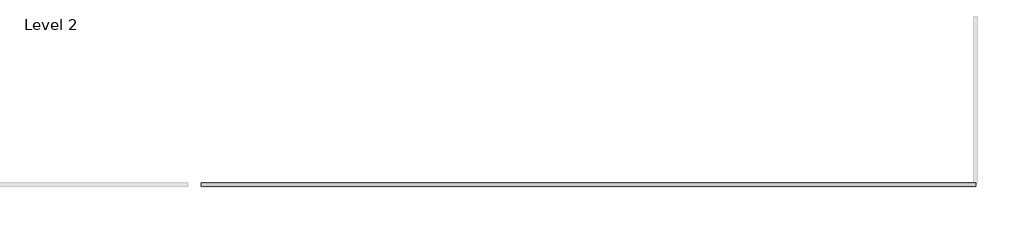
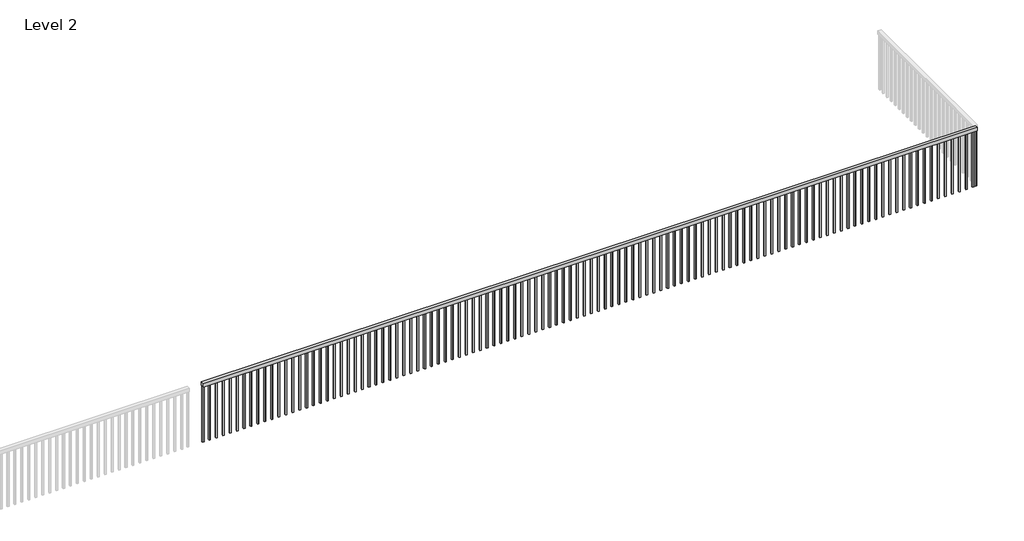
# One storey, part 2 of 5: 1 railing.
"""IFC4 building model written with IfcOpenShell, lengths in millimetres."""

from ifc_helpers import new_model, si_unit, frame, origin, place, context, project, spatial, polyline, outline, extrude, element, save

model = new_model("IFC4")

# Units and contexts
model_context = context("Model", 3, world=origin())
ifc_project = project(units=[si_unit("LENGTHUNIT", "METRE", prefix="MILLI")], contexts=[model_context])

# Site, building, storey
site = spatial("IfcSite", under=ifc_project)
building = spatial("IfcBuilding", under=site)
storey = spatial("IfcBuildingStorey", under=building, Name="Level 2", Elevation=3048.0)

# Railing
placement = place(None, origin())
element("IfcRailing", 1, ObjectType="Handrail - Rectangular", at=placement, inside=storey, context=model_context, shape_type="SweptSolid", body=[
    extrude(outline(polyline([(2981.3361222, -12911.7749501), (2981.3361222, -12860.9749501), (14309.7361222, -12860.9749501), (14309.7361222, -12911.7749501), (2981.3361222, -12911.7749501)])), frame((0.0, 0.0, 3911.6), z_axis=(0.0, 0.0, 1.0), x_axis=(1.0, 0.0, 0.0)), (0.0, 0.0, 1.0), 50.8),
    extrude(outline(polyline([(14249.4111222, -12895.8999501), (14249.4111222, -12876.8499501), (14268.4611222, -12876.8499501), (14268.4611222, -12895.8999501), (14249.4111222, -12895.8999501)])), frame((0.0, 0.0, 3048.0), z_axis=(0.0, 0.0, 1.0), x_axis=(1.0, 0.0, 0.0)), (0.0, 0.0, 1.0), 863.6),
    extrude(outline(polyline([(14147.8111222, -12895.8999501), (14147.8111222, -12876.8499501), (14166.8611222, -12876.8499501), (14166.8611222, -12895.8999501), (14147.8111222, -12895.8999501)])), frame((0.0, 0.0, 3048.0), z_axis=(0.0, 0.0, 1.0), x_axis=(1.0, 0.0, 0.0)), (0.0, 0.0, 1.0), 863.6),
    extrude(outline(polyline([(14046.2111222, -12895.8999501), (14046.2111222, -12876.8499501), (14065.2611222, -12876.8499501), (14065.2611222, -12895.8999501), (14046.2111222, -12895.8999501)])), frame((0.0, 0.0, 3048.0), z_axis=(0.0, 0.0, 1.0), x_axis=(1.0, 0.0, 0.0)), (0.0, 0.0, 1.0), 863.6),
    extrude(outline(polyline([(13944.6111222, -12895.8999501), (13944.6111222, -12876.8499501), (13963.6611222, -12876.8499501), (13963.6611222, -12895.8999501), (13944.6111222, -12895.8999501)])), frame((0.0, 0.0, 3048.0), z_axis=(0.0, 0.0, 1.0), x_axis=(1.0, 0.0, 0.0)), (0.0, 0.0, 1.0), 863.6),
    extrude(outline(polyline([(13843.0111222, -12895.8999501), (13843.0111222, -12876.8499501), (13862.0611222, -12876.8499501), (13862.0611222, -12895.8999501), (13843.0111222, -12895.8999501)])), frame((0.0, 0.0, 3048.0), z_axis=(0.0, 0.0, 1.0), x_axis=(1.0, 0.0, 0.0)), (0.0, 0.0, 1.0), 863.6),
    extrude(outline(polyline([(13741.4111222, -12895.8999501), (13741.4111222, -12876.8499501), (13760.4611222, -12876.8499501), (13760.4611222, -12895.8999501), (13741.4111222, -12895.8999501)])), frame((0.0, 0.0, 3048.0), z_axis=(0.0, 0.0, 1.0), x_axis=(1.0, 0.0, 0.0)), (0.0, 0.0, 1.0), 863.6),
    extrude(outline(polyline([(13639.8111222, -12895.8999501), (13639.8111222, -12876.8499501), (13658.8611222, -12876.8499501), (13658.8611222, -12895.8999501), (13639.8111222, -12895.8999501)])), frame((0.0, 0.0, 3048.0), z_axis=(0.0, 0.0, 1.0), x_axis=(1.0, 0.0, 0.0)), (0.0, 0.0, 1.0), 863.6),
    extrude(outline(polyline([(13538.2111222, -12895.8999501), (13538.2111222, -12876.8499501), (13557.2611222, -12876.8499501), (13557.2611222, -12895.8999501), (13538.2111222, -12895.8999501)])), frame((0.0, 0.0, 3048.0), z_axis=(0.0, 0.0, 1.0), x_axis=(1.0, 0.0, 0.0)), (0.0, 0.0, 1.0), 863.6),
    extrude(outline(polyline([(13436.6111222, -12895.8999501), (13436.6111222, -12876.8499501), (13455.6611222, -12876.8499501), (13455.6611222, -12895.8999501), (13436.6111222, -12895.8999501)])), frame((0.0, 0.0, 3048.0), z_axis=(0.0, 0.0, 1.0), x_axis=(1.0, 0.0, 0.0)), (0.0, 0.0, 1.0), 863.6),
    extrude(outline(polyline([(13335.0111222, -12895.8999501), (13335.0111222, -12876.8499501), (13354.0611222, -12876.8499501), (13354.0611222, -12895.8999501), (13335.0111222, -12895.8999501)])), frame((0.0, 0.0, 3048.0), z_axis=(0.0, 0.0, 1.0), x_axis=(1.0, 0.0, 0.0)), (0.0, 0.0, 1.0), 863.6),
    extrude(outline(polyline([(13233.4111222, -12895.8999501), (13233.4111222, -12876.8499501), (13252.4611222, -12876.8499501), (13252.4611222, -12895.8999501), (13233.4111222, -12895.8999501)])), frame((0.0, 0.0, 3048.0), z_axis=(0.0, 0.0, 1.0), x_axis=(1.0, 0.0, 0.0)), (0.0, 0.0, 1.0), 863.6),
    extrude(outline(polyline([(13131.8111222, -12895.8999501), (13131.8111222, -12876.8499501), (13150.8611222, -12876.8499501), (13150.8611222, -12895.8999501), (13131.8111222, -12895.8999501)])), frame((0.0, 0.0, 3048.0), z_axis=(0.0, 0.0, 1.0), x_axis=(1.0, 0.0, 0.0)), (0.0, 0.0, 1.0), 863.6),
    extrude(outline(polyline([(13030.2111222, -12895.8999501), (13030.2111222, -12876.8499501), (13049.2611222, -12876.8499501), (13049.2611222, -12895.8999501), (13030.2111222, -12895.8999501)])), frame((0.0, 0.0, 3048.0), z_axis=(0.0, 0.0, 1.0), x_axis=(1.0, 0.0, 0.0)), (0.0, 0.0, 1.0), 863.6),
    extrude(outline(polyline([(12928.6111222, -12895.8999501), (12928.6111222, -12876.8499501), (12947.6611222, -12876.8499501), (12947.6611222, -12895.8999501), (12928.6111222, -12895.8999501)])), frame((0.0, 0.0, 3048.0), z_axis=(0.0, 0.0, 1.0), x_axis=(1.0, 0.0, 0.0)), (0.0, 0.0, 1.0), 863.6),
    extrude(outline(polyline([(12827.0111222, -12895.8999501), (12827.0111222, -12876.8499501), (12846.0611222, -12876.8499501), (12846.0611222, -12895.8999501), (12827.0111222, -12895.8999501)])), frame((0.0, 0.0, 3048.0), z_axis=(0.0, 0.0, 1.0), x_axis=(1.0, 0.0, 0.0)), (0.0, 0.0, 1.0), 863.6),
    extrude(outline(polyline([(12725.4111222, -12895.8999501), (12725.4111222, -12876.8499501), (12744.4611222, -12876.8499501), (12744.4611222, -12895.8999501), (12725.4111222, -12895.8999501)])), frame((0.0, 0.0, 3048.0), z_axis=(0.0, 0.0, 1.0), x_axis=(1.0, 0.0, 0.0)), (0.0, 0.0, 1.0), 863.6),
    extrude(outline(polyline([(12623.8111222, -12895.8999501), (12623.8111222, -12876.8499501), (12642.8611222, -12876.8499501), (12642.8611222, -12895.8999501), (12623.8111222, -12895.8999501)])), frame((0.0, 0.0, 3048.0), z_axis=(0.0, 0.0, 1.0), x_axis=(1.0, 0.0, 0.0)), (0.0, 0.0, 1.0), 863.6),
    extrude(outline(polyline([(12522.2111222, -12895.8999501), (12522.2111222, -12876.8499501), (12541.2611222, -12876.8499501), (12541.2611222, -12895.8999501), (12522.2111222, -12895.8999501)])), frame((0.0, 0.0, 3048.0), z_axis=(0.0, 0.0, 1.0), x_axis=(1.0, 0.0, 0.0)), (0.0, 0.0, 1.0), 863.6),
    extrude(outline(polyline([(12420.6111222, -12895.8999501), (12420.6111222, -12876.8499501), (12439.6611222, -12876.8499501), (12439.6611222, -12895.8999501), (12420.6111222, -12895.8999501)])), frame((0.0, 0.0, 3048.0), z_axis=(0.0, 0.0, 1.0), x_axis=(1.0, 0.0, 0.0)), (0.0, 0.0, 1.0), 863.6),
    extrude(outline(polyline([(12319.0111222, -12895.8999501), (12319.0111222, -12876.8499501), (12338.0611222, -12876.8499501), (12338.0611222, -12895.8999501), (12319.0111222, -12895.8999501)])), frame((0.0, 0.0, 3048.0), z_axis=(0.0, 0.0, 1.0), x_axis=(1.0, 0.0, 0.0)), (0.0, 0.0, 1.0), 863.6),
    extrude(outline(polyline([(12217.4111222, -12895.8999501), (12217.4111222, -12876.8499501), (12236.4611222, -12876.8499501), (12236.4611222, -12895.8999501), (12217.4111222, -12895.8999501)])), frame((0.0, 0.0, 3048.0), z_axis=(0.0, 0.0, 1.0), x_axis=(1.0, 0.0, 0.0)), (0.0, 0.0, 1.0), 863.6),
    extrude(outline(polyline([(12115.8111222, -12895.8999501), (12115.8111222, -12876.8499501), (12134.8611222, -12876.8499501), (12134.8611222, -12895.8999501), (12115.8111222, -12895.8999501)])), frame((0.0, 0.0, 3048.0), z_axis=(0.0, 0.0, 1.0), x_axis=(1.0, 0.0, 0.0)), (0.0, 0.0, 1.0), 863.6),
    extrude(outline(polyline([(12014.2111222, -12895.8999501), (12014.2111222, -12876.8499501), (12033.2611222, -12876.8499501), (12033.2611222, -12895.8999501), (12014.2111222, -12895.8999501)])), frame((0.0, 0.0, 3048.0), z_axis=(0.0, 0.0, 1.0), x_axis=(1.0, 0.0, 0.0)), (0.0, 0.0, 1.0), 863.6),
    extrude(outline(polyline([(11912.6111222, -12895.8999501), (11912.6111222, -12876.8499501), (11931.6611222, -12876.8499501), (11931.6611222, -12895.8999501), (11912.6111222, -12895.8999501)])), frame((0.0, 0.0, 3048.0), z_axis=(0.0, 0.0, 1.0), x_axis=(1.0, 0.0, 0.0)), (0.0, 0.0, 1.0), 863.6),
    extrude(outline(polyline([(11811.0111222, -12895.8999501), (11811.0111222, -12876.8499501), (11830.0611222, -12876.8499501), (11830.0611222, -12895.8999501), (11811.0111222, -12895.8999501)])), frame((0.0, 0.0, 3048.0), z_axis=(0.0, 0.0, 1.0), x_axis=(1.0, 0.0, 0.0)), (0.0, 0.0, 1.0), 863.6),
    extrude(outline(polyline([(11709.4111222, -12895.8999501), (11709.4111222, -12876.8499501), (11728.4611222, -12876.8499501), (11728.4611222, -12895.8999501), (11709.4111222, -12895.8999501)])), frame((0.0, 0.0, 3048.0), z_axis=(0.0, 0.0, 1.0), x_axis=(1.0, 0.0, 0.0)), (0.0, 0.0, 1.0), 863.6),
    extrude(outline(polyline([(11607.8111222, -12895.8999501), (11607.8111222, -12876.8499501), (11626.8611222, -12876.8499501), (11626.8611222, -12895.8999501), (11607.8111222, -12895.8999501)])), frame((0.0, 0.0, 3048.0), z_axis=(0.0, 0.0, 1.0), x_axis=(1.0, 0.0, 0.0)), (0.0, 0.0, 1.0), 863.6),
    extrude(outline(polyline([(11506.2111222, -12895.8999501), (11506.2111222, -12876.8499501), (11525.2611222, -12876.8499501), (11525.2611222, -12895.8999501), (11506.2111222, -12895.8999501)])), frame((0.0, 0.0, 3048.0), z_axis=(0.0, 0.0, 1.0), x_axis=(1.0, 0.0, 0.0)), (0.0, 0.0, 1.0), 863.6),
    extrude(outline(polyline([(11404.6111222, -12895.8999501), (11404.6111222, -12876.8499501), (11423.6611222, -12876.8499501), (11423.6611222, -12895.8999501), (11404.6111222, -12895.8999501)])), frame((0.0, 0.0, 3048.0), z_axis=(0.0, 0.0, 1.0), x_axis=(1.0, 0.0, 0.0)), (0.0, 0.0, 1.0), 863.6),
    extrude(outline(polyline([(11303.0111222, -12895.8999501), (11303.0111222, -12876.8499501), (11322.0611222, -12876.8499501), (11322.0611222, -12895.8999501), (11303.0111222, -12895.8999501)])), frame((0.0, 0.0, 3048.0), z_axis=(0.0, 0.0, 1.0), x_axis=(1.0, 0.0, 0.0)), (0.0, 0.0, 1.0), 863.6),
    extrude(outline(polyline([(11201.4111222, -12895.8999501), (11201.4111222, -12876.8499501), (11220.4611222, -12876.8499501), (11220.4611222, -12895.8999501), (11201.4111222, -12895.8999501)])), frame((0.0, 0.0, 3048.0), z_axis=(0.0, 0.0, 1.0), x_axis=(1.0, 0.0, 0.0)), (0.0, 0.0, 1.0), 863.6),
    extrude(outline(polyline([(11099.8111222, -12895.8999501), (11099.8111222, -12876.8499501), (11118.8611222, -12876.8499501), (11118.8611222, -12895.8999501), (11099.8111222, -12895.8999501)])), frame((0.0, 0.0, 3048.0), z_axis=(0.0, 0.0, 1.0), x_axis=(1.0, 0.0, 0.0)), (0.0, 0.0, 1.0), 863.6),
    extrude(outline(polyline([(10998.2111222, -12895.8999501), (10998.2111222, -12876.8499501), (11017.2611222, -12876.8499501), (11017.2611222, -12895.8999501), (10998.2111222, -12895.8999501)])), frame((0.0, 0.0, 3048.0), z_axis=(0.0, 0.0, 1.0), x_axis=(1.0, 0.0, 0.0)), (0.0, 0.0, 1.0), 863.6),
    extrude(outline(polyline([(10896.6111222, -12895.8999501), (10896.6111222, -12876.8499501), (10915.6611222, -12876.8499501), (10915.6611222, -12895.8999501), (10896.6111222, -12895.8999501)])), frame((0.0, 0.0, 3048.0), z_axis=(0.0, 0.0, 1.0), x_axis=(1.0, 0.0, 0.0)), (0.0, 0.0, 1.0), 863.6),
    extrude(outline(polyline([(10795.0111222, -12895.8999501), (10795.0111222, -12876.8499501), (10814.0611222, -12876.8499501), (10814.0611222, -12895.8999501), (10795.0111222, -12895.8999501)])), frame((0.0, 0.0, 3048.0), z_axis=(0.0, 0.0, 1.0), x_axis=(1.0, 0.0, 0.0)), (0.0, 0.0, 1.0), 863.6),
    extrude(outline(polyline([(10693.4111222, -12895.8999501), (10693.4111222, -12876.8499501), (10712.4611222, -12876.8499501), (10712.4611222, -12895.8999501), (10693.4111222, -12895.8999501)])), frame((0.0, 0.0, 3048.0), z_axis=(0.0, 0.0, 1.0), x_axis=(1.0, 0.0, 0.0)), (0.0, 0.0, 1.0), 863.6),
    extrude(outline(polyline([(10591.8111222, -12895.8999501), (10591.8111222, -12876.8499501), (10610.8611222, -12876.8499501), (10610.8611222, -12895.8999501), (10591.8111222, -12895.8999501)])), frame((0.0, 0.0, 3048.0), z_axis=(0.0, 0.0, 1.0), x_axis=(1.0, 0.0, 0.0)), (0.0, 0.0, 1.0), 863.6),
    extrude(outline(polyline([(10490.2111222, -12895.8999501), (10490.2111222, -12876.8499501), (10509.2611222, -12876.8499501), (10509.2611222, -12895.8999501), (10490.2111222, -12895.8999501)])), frame((0.0, 0.0, 3048.0), z_axis=(0.0, 0.0, 1.0), x_axis=(1.0, 0.0, 0.0)), (0.0, 0.0, 1.0), 863.6),
    extrude(outline(polyline([(10388.6111222, -12895.8999501), (10388.6111222, -12876.8499501), (10407.6611222, -12876.8499501), (10407.6611222, -12895.8999501), (10388.6111222, -12895.8999501)])), frame((0.0, 0.0, 3048.0), z_axis=(0.0, 0.0, 1.0), x_axis=(1.0, 0.0, 0.0)), (0.0, 0.0, 1.0), 863.6),
    extrude(outline(polyline([(10287.0111222, -12895.8999501), (10287.0111222, -12876.8499501), (10306.0611222, -12876.8499501), (10306.0611222, -12895.8999501), (10287.0111222, -12895.8999501)])), frame((0.0, 0.0, 3048.0), z_axis=(0.0, 0.0, 1.0), x_axis=(1.0, 0.0, 0.0)), (0.0, 0.0, 1.0), 863.6),
    extrude(outline(polyline([(10185.4111222, -12895.8999501), (10185.4111222, -12876.8499501), (10204.4611222, -12876.8499501), (10204.4611222, -12895.8999501), (10185.4111222, -12895.8999501)])), frame((0.0, 0.0, 3048.0), z_axis=(0.0, 0.0, 1.0), x_axis=(1.0, 0.0, 0.0)), (0.0, 0.0, 1.0), 863.6),
    extrude(outline(polyline([(10083.8111222, -12895.8999501), (10083.8111222, -12876.8499501), (10102.8611222, -12876.8499501), (10102.8611222, -12895.8999501), (10083.8111222, -12895.8999501)])), frame((0.0, 0.0, 3048.0), z_axis=(0.0, 0.0, 1.0), x_axis=(1.0, 0.0, 0.0)), (0.0, 0.0, 1.0), 863.6),
    extrude(outline(polyline([(9982.2111222, -12895.8999501), (9982.2111222, -12876.8499501), (10001.2611222, -12876.8499501), (10001.2611222, -12895.8999501), (9982.2111222, -12895.8999501)])), frame((0.0, 0.0, 3048.0), z_axis=(0.0, 0.0, 1.0), x_axis=(1.0, 0.0, 0.0)), (0.0, 0.0, 1.0), 863.6),
    extrude(outline(polyline([(9880.6111222, -12895.8999501), (9880.6111222, -12876.8499501), (9899.6611222, -12876.8499501), (9899.6611222, -12895.8999501), (9880.6111222, -12895.8999501)])), frame((0.0, 0.0, 3048.0), z_axis=(0.0, 0.0, 1.0), x_axis=(1.0, 0.0, 0.0)), (0.0, 0.0, 1.0), 863.6),
    extrude(outline(polyline([(9779.0111222, -12895.8999501), (9779.0111222, -12876.8499501), (9798.0611222, -12876.8499501), (9798.0611222, -12895.8999501), (9779.0111222, -12895.8999501)])), frame((0.0, 0.0, 3048.0), z_axis=(0.0, 0.0, 1.0), x_axis=(1.0, 0.0, 0.0)), (0.0, 0.0, 1.0), 863.6),
    extrude(outline(polyline([(9677.4111222, -12895.8999501), (9677.4111222, -12876.8499501), (9696.4611222, -12876.8499501), (9696.4611222, -12895.8999501), (9677.4111222, -12895.8999501)])), frame((0.0, 0.0, 3048.0), z_axis=(0.0, 0.0, 1.0), x_axis=(1.0, 0.0, 0.0)), (0.0, 0.0, 1.0), 863.6),
    extrude(outline(polyline([(9575.8111222, -12895.8999501), (9575.8111222, -12876.8499501), (9594.8611222, -12876.8499501), (9594.8611222, -12895.8999501), (9575.8111222, -12895.8999501)])), frame((0.0, 0.0, 3048.0), z_axis=(0.0, 0.0, 1.0), x_axis=(1.0, 0.0, 0.0)), (0.0, 0.0, 1.0), 863.6),
    extrude(outline(polyline([(9474.2111222, -12895.8999501), (9474.2111222, -12876.8499501), (9493.2611222, -12876.8499501), (9493.2611222, -12895.8999501), (9474.2111222, -12895.8999501)])), frame((0.0, 0.0, 3048.0), z_axis=(0.0, 0.0, 1.0), x_axis=(1.0, 0.0, 0.0)), (0.0, 0.0, 1.0), 863.6),
    extrude(outline(polyline([(9372.6111222, -12895.8999501), (9372.6111222, -12876.8499501), (9391.6611222, -12876.8499501), (9391.6611222, -12895.8999501), (9372.6111222, -12895.8999501)])), frame((0.0, 0.0, 3048.0), z_axis=(0.0, 0.0, 1.0), x_axis=(1.0, 0.0, 0.0)), (0.0, 0.0, 1.0), 863.6),
    extrude(outline(polyline([(9271.0111222, -12895.8999501), (9271.0111222, -12876.8499501), (9290.0611222, -12876.8499501), (9290.0611222, -12895.8999501), (9271.0111222, -12895.8999501)])), frame((0.0, 0.0, 3048.0), z_axis=(0.0, 0.0, 1.0), x_axis=(1.0, 0.0, 0.0)), (0.0, 0.0, 1.0), 863.6),
    extrude(outline(polyline([(9169.4111222, -12895.8999501), (9169.4111222, -12876.8499501), (9188.4611222, -12876.8499501), (9188.4611222, -12895.8999501), (9169.4111222, -12895.8999501)])), frame((0.0, 0.0, 3048.0), z_axis=(0.0, 0.0, 1.0), x_axis=(1.0, 0.0, 0.0)), (0.0, 0.0, 1.0), 863.6),
    extrude(outline(polyline([(9067.8111222, -12895.8999501), (9067.8111222, -12876.8499501), (9086.8611222, -12876.8499501), (9086.8611222, -12895.8999501), (9067.8111222, -12895.8999501)])), frame((0.0, 0.0, 3048.0), z_axis=(0.0, 0.0, 1.0), x_axis=(1.0, 0.0, 0.0)), (0.0, 0.0, 1.0), 863.6),
    extrude(outline(polyline([(8966.2111222, -12895.8999501), (8966.2111222, -12876.8499501), (8985.2611222, -12876.8499501), (8985.2611222, -12895.8999501), (8966.2111222, -12895.8999501)])), frame((0.0, 0.0, 3048.0), z_axis=(0.0, 0.0, 1.0), x_axis=(1.0, 0.0, 0.0)), (0.0, 0.0, 1.0), 863.6),
    extrude(outline(polyline([(8864.6111222, -12895.8999501), (8864.6111222, -12876.8499501), (8883.6611222, -12876.8499501), (8883.6611222, -12895.8999501), (8864.6111222, -12895.8999501)])), frame((0.0, 0.0, 3048.0), z_axis=(0.0, 0.0, 1.0), x_axis=(1.0, 0.0, 0.0)), (0.0, 0.0, 1.0), 863.6),
    extrude(outline(polyline([(8763.0111222, -12895.8999501), (8763.0111222, -12876.8499501), (8782.0611222, -12876.8499501), (8782.0611222, -12895.8999501), (8763.0111222, -12895.8999501)])), frame((0.0, 0.0, 3048.0), z_axis=(0.0, 0.0, 1.0), x_axis=(1.0, 0.0, 0.0)), (0.0, 0.0, 1.0), 863.6),
    extrude(outline(polyline([(8661.4111222, -12895.8999501), (8661.4111222, -12876.8499501), (8680.4611222, -12876.8499501), (8680.4611222, -12895.8999501), (8661.4111222, -12895.8999501)])), frame((0.0, 0.0, 3048.0), z_axis=(0.0, 0.0, 1.0), x_axis=(1.0, 0.0, 0.0)), (0.0, 0.0, 1.0), 863.6),
    extrude(outline(polyline([(8559.8111222, -12895.8999501), (8559.8111222, -12876.8499501), (8578.8611222, -12876.8499501), (8578.8611222, -12895.8999501), (8559.8111222, -12895.8999501)])), frame((0.0, 0.0, 3048.0), z_axis=(0.0, 0.0, 1.0), x_axis=(1.0, 0.0, 0.0)), (0.0, 0.0, 1.0), 863.6),
    extrude(outline(polyline([(8458.2111222, -12895.8999501), (8458.2111222, -12876.8499501), (8477.2611222, -12876.8499501), (8477.2611222, -12895.8999501), (8458.2111222, -12895.8999501)])), frame((0.0, 0.0, 3048.0), z_axis=(0.0, 0.0, 1.0), x_axis=(1.0, 0.0, 0.0)), (0.0, 0.0, 1.0), 863.6),
    extrude(outline(polyline([(8356.6111222, -12895.8999501), (8356.6111222, -12876.8499501), (8375.6611222, -12876.8499501), (8375.6611222, -12895.8999501), (8356.6111222, -12895.8999501)])), frame((0.0, 0.0, 3048.0), z_axis=(0.0, 0.0, 1.0), x_axis=(1.0, 0.0, 0.0)), (0.0, 0.0, 1.0), 863.6),
    extrude(outline(polyline([(8255.0111222, -12895.8999501), (8255.0111222, -12876.8499501), (8274.0611222, -12876.8499501), (8274.0611222, -12895.8999501), (8255.0111222, -12895.8999501)])), frame((0.0, 0.0, 3048.0), z_axis=(0.0, 0.0, 1.0), x_axis=(1.0, 0.0, 0.0)), (0.0, 0.0, 1.0), 863.6),
    extrude(outline(polyline([(8153.4111222, -12895.8999501), (8153.4111222, -12876.8499501), (8172.4611222, -12876.8499501), (8172.4611222, -12895.8999501), (8153.4111222, -12895.8999501)])), frame((0.0, 0.0, 3048.0), z_axis=(0.0, 0.0, 1.0), x_axis=(1.0, 0.0, 0.0)), (0.0, 0.0, 1.0), 863.6),
    extrude(outline(polyline([(8051.8111222, -12895.8999501), (8051.8111222, -12876.8499501), (8070.8611222, -12876.8499501), (8070.8611222, -12895.8999501), (8051.8111222, -12895.8999501)])), frame((0.0, 0.0, 3048.0), z_axis=(0.0, 0.0, 1.0), x_axis=(1.0, 0.0, 0.0)), (0.0, 0.0, 1.0), 863.6),
    extrude(outline(polyline([(7950.2111222, -12895.8999501), (7950.2111222, -12876.8499501), (7969.2611222, -12876.8499501), (7969.2611222, -12895.8999501), (7950.2111222, -12895.8999501)])), frame((0.0, 0.0, 3048.0), z_axis=(0.0, 0.0, 1.0), x_axis=(1.0, 0.0, 0.0)), (0.0, 0.0, 1.0), 863.6),
    extrude(outline(polyline([(7848.6111222, -12895.8999501), (7848.6111222, -12876.8499501), (7867.6611222, -12876.8499501), (7867.6611222, -12895.8999501), (7848.6111222, -12895.8999501)])), frame((0.0, 0.0, 3048.0), z_axis=(0.0, 0.0, 1.0), x_axis=(1.0, 0.0, 0.0)), (0.0, 0.0, 1.0), 863.6),
    extrude(outline(polyline([(7747.0111222, -12895.8999501), (7747.0111222, -12876.8499501), (7766.0611222, -12876.8499501), (7766.0611222, -12895.8999501), (7747.0111222, -12895.8999501)])), frame((0.0, 0.0, 3048.0), z_axis=(0.0, 0.0, 1.0), x_axis=(1.0, 0.0, 0.0)), (0.0, 0.0, 1.0), 863.6),
    extrude(outline(polyline([(7645.4111222, -12895.8999501), (7645.4111222, -12876.8499501), (7664.4611222, -12876.8499501), (7664.4611222, -12895.8999501), (7645.4111222, -12895.8999501)])), frame((0.0, 0.0, 3048.0), z_axis=(0.0, 0.0, 1.0), x_axis=(1.0, 0.0, 0.0)), (0.0, 0.0, 1.0), 863.6),
    extrude(outline(polyline([(7543.8111222, -12895.8999501), (7543.8111222, -12876.8499501), (7562.8611222, -12876.8499501), (7562.8611222, -12895.8999501), (7543.8111222, -12895.8999501)])), frame((0.0, 0.0, 3048.0), z_axis=(0.0, 0.0, 1.0), x_axis=(1.0, 0.0, 0.0)), (0.0, 0.0, 1.0), 863.6),
    extrude(outline(polyline([(7442.2111222, -12895.8999501), (7442.2111222, -12876.8499501), (7461.2611222, -12876.8499501), (7461.2611222, -12895.8999501), (7442.2111222, -12895.8999501)])), frame((0.0, 0.0, 3048.0), z_axis=(0.0, 0.0, 1.0), x_axis=(1.0, 0.0, 0.0)), (0.0, 0.0, 1.0), 863.6),
    extrude(outline(polyline([(7340.6111222, -12895.8999501), (7340.6111222, -12876.8499501), (7359.6611222, -12876.8499501), (7359.6611222, -12895.8999501), (7340.6111222, -12895.8999501)])), frame((0.0, 0.0, 3048.0), z_axis=(0.0, 0.0, 1.0), x_axis=(1.0, 0.0, 0.0)), (0.0, 0.0, 1.0), 863.6),
    extrude(outline(polyline([(7239.0111222, -12895.8999501), (7239.0111222, -12876.8499501), (7258.0611222, -12876.8499501), (7258.0611222, -12895.8999501), (7239.0111222, -12895.8999501)])), frame((0.0, 0.0, 3048.0), z_axis=(0.0, 0.0, 1.0), x_axis=(1.0, 0.0, 0.0)), (0.0, 0.0, 1.0), 863.6),
    extrude(outline(polyline([(7137.4111222, -12895.8999501), (7137.4111222, -12876.8499501), (7156.4611222, -12876.8499501), (7156.4611222, -12895.8999501), (7137.4111222, -12895.8999501)])), frame((0.0, 0.0, 3048.0), z_axis=(0.0, 0.0, 1.0), x_axis=(1.0, 0.0, 0.0)), (0.0, 0.0, 1.0), 863.6),
    extrude(outline(polyline([(7035.8111222, -12895.8999501), (7035.8111222, -12876.8499501), (7054.8611222, -12876.8499501), (7054.8611222, -12895.8999501), (7035.8111222, -12895.8999501)])), frame((0.0, 0.0, 3048.0), z_axis=(0.0, 0.0, 1.0), x_axis=(1.0, 0.0, 0.0)), (0.0, 0.0, 1.0), 863.6),
    extrude(outline(polyline([(6934.2111222, -12895.8999501), (6934.2111222, -12876.8499501), (6953.2611222, -12876.8499501), (6953.2611222, -12895.8999501), (6934.2111222, -12895.8999501)])), frame((0.0, 0.0, 3048.0), z_axis=(0.0, 0.0, 1.0), x_axis=(1.0, 0.0, 0.0)), (0.0, 0.0, 1.0), 863.6),
    extrude(outline(polyline([(6832.6111222, -12895.8999501), (6832.6111222, -12876.8499501), (6851.6611222, -12876.8499501), (6851.6611222, -12895.8999501), (6832.6111222, -12895.8999501)])), frame((0.0, 0.0, 3048.0), z_axis=(0.0, 0.0, 1.0), x_axis=(1.0, 0.0, 0.0)), (0.0, 0.0, 1.0), 863.6),
    extrude(outline(polyline([(6731.0111222, -12895.8999501), (6731.0111222, -12876.8499501), (6750.0611222, -12876.8499501), (6750.0611222, -12895.8999501), (6731.0111222, -12895.8999501)])), frame((0.0, 0.0, 3048.0), z_axis=(0.0, 0.0, 1.0), x_axis=(1.0, 0.0, 0.0)), (0.0, 0.0, 1.0), 863.6),
    extrude(outline(polyline([(6629.4111222, -12895.8999501), (6629.4111222, -12876.8499501), (6648.4611222, -12876.8499501), (6648.4611222, -12895.8999501), (6629.4111222, -12895.8999501)])), frame((0.0, 0.0, 3048.0), z_axis=(0.0, 0.0, 1.0), x_axis=(1.0, 0.0, 0.0)), (0.0, 0.0, 1.0), 863.6),
    extrude(outline(polyline([(6527.8111222, -12895.8999501), (6527.8111222, -12876.8499501), (6546.8611222, -12876.8499501), (6546.8611222, -12895.8999501), (6527.8111222, -12895.8999501)])), frame((0.0, 0.0, 3048.0), z_axis=(0.0, 0.0, 1.0), x_axis=(1.0, 0.0, 0.0)), (0.0, 0.0, 1.0), 863.6),
    extrude(outline(polyline([(6426.2111222, -12895.8999501), (6426.2111222, -12876.8499501), (6445.2611222, -12876.8499501), (6445.2611222, -12895.8999501), (6426.2111222, -12895.8999501)])), frame((0.0, 0.0, 3048.0), z_axis=(0.0, 0.0, 1.0), x_axis=(1.0, 0.0, 0.0)), (0.0, 0.0, 1.0), 863.6),
    extrude(outline(polyline([(6324.6111222, -12895.8999501), (6324.6111222, -12876.8499501), (6343.6611222, -12876.8499501), (6343.6611222, -12895.8999501), (6324.6111222, -12895.8999501)])), frame((0.0, 0.0, 3048.0), z_axis=(0.0, 0.0, 1.0), x_axis=(1.0, 0.0, 0.0)), (0.0, 0.0, 1.0), 863.6),
    extrude(outline(polyline([(6223.0111222, -12895.8999501), (6223.0111222, -12876.8499501), (6242.0611222, -12876.8499501), (6242.0611222, -12895.8999501), (6223.0111222, -12895.8999501)])), frame((0.0, 0.0, 3048.0), z_axis=(0.0, 0.0, 1.0), x_axis=(1.0, 0.0, 0.0)), (0.0, 0.0, 1.0), 863.6),
    extrude(outline(polyline([(6121.4111222, -12895.8999501), (6121.4111222, -12876.8499501), (6140.4611222, -12876.8499501), (6140.4611222, -12895.8999501), (6121.4111222, -12895.8999501)])), frame((0.0, 0.0, 3048.0), z_axis=(0.0, 0.0, 1.0), x_axis=(1.0, 0.0, 0.0)), (0.0, 0.0, 1.0), 863.6),
    extrude(outline(polyline([(6019.8111222, -12895.8999501), (6019.8111222, -12876.8499501), (6038.8611222, -12876.8499501), (6038.8611222, -12895.8999501), (6019.8111222, -12895.8999501)])), frame((0.0, 0.0, 3048.0), z_axis=(0.0, 0.0, 1.0), x_axis=(1.0, 0.0, 0.0)), (0.0, 0.0, 1.0), 863.6),
    extrude(outline(polyline([(5918.2111222, -12895.8999501), (5918.2111222, -12876.8499501), (5937.2611222, -12876.8499501), (5937.2611222, -12895.8999501), (5918.2111222, -12895.8999501)])), frame((0.0, 0.0, 3048.0), z_axis=(0.0, 0.0, 1.0), x_axis=(1.0, 0.0, 0.0)), (0.0, 0.0, 1.0), 863.6),
    extrude(outline(polyline([(5816.6111222, -12895.8999501), (5816.6111222, -12876.8499501), (5835.6611222, -12876.8499501), (5835.6611222, -12895.8999501), (5816.6111222, -12895.8999501)])), frame((0.0, 0.0, 3048.0), z_axis=(0.0, 0.0, 1.0), x_axis=(1.0, 0.0, 0.0)), (0.0, 0.0, 1.0), 863.6),
    extrude(outline(polyline([(5715.0111222, -12895.8999501), (5715.0111222, -12876.8499501), (5734.0611222, -12876.8499501), (5734.0611222, -12895.8999501), (5715.0111222, -12895.8999501)])), frame((0.0, 0.0, 3048.0), z_axis=(0.0, 0.0, 1.0), x_axis=(1.0, 0.0, 0.0)), (0.0, 0.0, 1.0), 863.6),
    extrude(outline(polyline([(5613.4111222, -12895.8999501), (5613.4111222, -12876.8499501), (5632.4611222, -12876.8499501), (5632.4611222, -12895.8999501), (5613.4111222, -12895.8999501)])), frame((0.0, 0.0, 3048.0), z_axis=(0.0, 0.0, 1.0), x_axis=(1.0, 0.0, 0.0)), (0.0, 0.0, 1.0), 863.6),
    extrude(outline(polyline([(5511.8111222, -12895.8999501), (5511.8111222, -12876.8499501), (5530.8611222, -12876.8499501), (5530.8611222, -12895.8999501), (5511.8111222, -12895.8999501)])), frame((0.0, 0.0, 3048.0), z_axis=(0.0, 0.0, 1.0), x_axis=(1.0, 0.0, 0.0)), (0.0, 0.0, 1.0), 863.6),
    extrude(outline(polyline([(5410.2111222, -12895.8999501), (5410.2111222, -12876.8499501), (5429.2611222, -12876.8499501), (5429.2611222, -12895.8999501), (5410.2111222, -12895.8999501)])), frame((0.0, 0.0, 3048.0), z_axis=(0.0, 0.0, 1.0), x_axis=(1.0, 0.0, 0.0)), (0.0, 0.0, 1.0), 863.6),
    extrude(outline(polyline([(5308.6111222, -12895.8999501), (5308.6111222, -12876.8499501), (5327.6611222, -12876.8499501), (5327.6611222, -12895.8999501), (5308.6111222, -12895.8999501)])), frame((0.0, 0.0, 3048.0), z_axis=(0.0, 0.0, 1.0), x_axis=(1.0, 0.0, 0.0)), (0.0, 0.0, 1.0), 863.6),
    extrude(outline(polyline([(5207.0111222, -12895.8999501), (5207.0111222, -12876.8499501), (5226.0611222, -12876.8499501), (5226.0611222, -12895.8999501), (5207.0111222, -12895.8999501)])), frame((0.0, 0.0, 3048.0), z_axis=(0.0, 0.0, 1.0), x_axis=(1.0, 0.0, 0.0)), (0.0, 0.0, 1.0), 863.6),
    extrude(outline(polyline([(5105.4111222, -12895.8999501), (5105.4111222, -12876.8499501), (5124.4611222, -12876.8499501), (5124.4611222, -12895.8999501), (5105.4111222, -12895.8999501)])), frame((0.0, 0.0, 3048.0), z_axis=(0.0, 0.0, 1.0), x_axis=(1.0, 0.0, 0.0)), (0.0, 0.0, 1.0), 863.6),
    extrude(outline(polyline([(5003.8111222, -12895.8999501), (5003.8111222, -12876.8499501), (5022.8611222, -12876.8499501), (5022.8611222, -12895.8999501), (5003.8111222, -12895.8999501)])), frame((0.0, 0.0, 3048.0), z_axis=(0.0, 0.0, 1.0), x_axis=(1.0, 0.0, 0.0)), (0.0, 0.0, 1.0), 863.6),
    extrude(outline(polyline([(4902.2111222, -12895.8999501), (4902.2111222, -12876.8499501), (4921.2611222, -12876.8499501), (4921.2611222, -12895.8999501), (4902.2111222, -12895.8999501)])), frame((0.0, 0.0, 3048.0), z_axis=(0.0, 0.0, 1.0), x_axis=(1.0, 0.0, 0.0)), (0.0, 0.0, 1.0), 863.6),
    extrude(outline(polyline([(4800.6111222, -12895.8999501), (4800.6111222, -12876.8499501), (4819.6611222, -12876.8499501), (4819.6611222, -12895.8999501), (4800.6111222, -12895.8999501)])), frame((0.0, 0.0, 3048.0), z_axis=(0.0, 0.0, 1.0), x_axis=(1.0, 0.0, 0.0)), (0.0, 0.0, 1.0), 863.6),
    extrude(outline(polyline([(4699.0111222, -12895.8999501), (4699.0111222, -12876.8499501), (4718.0611222, -12876.8499501), (4718.0611222, -12895.8999501), (4699.0111222, -12895.8999501)])), frame((0.0, 0.0, 3048.0), z_axis=(0.0, 0.0, 1.0), x_axis=(1.0, 0.0, 0.0)), (0.0, 0.0, 1.0), 863.6),
    extrude(outline(polyline([(4597.4111222, -12895.8999501), (4597.4111222, -12876.8499501), (4616.4611222, -12876.8499501), (4616.4611222, -12895.8999501), (4597.4111222, -12895.8999501)])), frame((0.0, 0.0, 3048.0), z_axis=(0.0, 0.0, 1.0), x_axis=(1.0, 0.0, 0.0)), (0.0, 0.0, 1.0), 863.6),
    extrude(outline(polyline([(4495.8111222, -12895.8999501), (4495.8111222, -12876.8499501), (4514.8611222, -12876.8499501), (4514.8611222, -12895.8999501), (4495.8111222, -12895.8999501)])), frame((0.0, 0.0, 3048.0), z_axis=(0.0, 0.0, 1.0), x_axis=(1.0, 0.0, 0.0)), (0.0, 0.0, 1.0), 863.6),
    extrude(outline(polyline([(4394.2111222, -12895.8999501), (4394.2111222, -12876.8499501), (4413.2611222, -12876.8499501), (4413.2611222, -12895.8999501), (4394.2111222, -12895.8999501)])), frame((0.0, 0.0, 3048.0), z_axis=(0.0, 0.0, 1.0), x_axis=(1.0, 0.0, 0.0)), (0.0, 0.0, 1.0), 863.6),
    extrude(outline(polyline([(4292.6111222, -12895.8999501), (4292.6111222, -12876.8499501), (4311.6611222, -12876.8499501), (4311.6611222, -12895.8999501), (4292.6111222, -12895.8999501)])), frame((0.0, 0.0, 3048.0), z_axis=(0.0, 0.0, 1.0), x_axis=(1.0, 0.0, 0.0)), (0.0, 0.0, 1.0), 863.6),
    extrude(outline(polyline([(4191.0111222, -12895.8999501), (4191.0111222, -12876.8499501), (4210.0611222, -12876.8499501), (4210.0611222, -12895.8999501), (4191.0111222, -12895.8999501)])), frame((0.0, 0.0, 3048.0), z_axis=(0.0, 0.0, 1.0), x_axis=(1.0, 0.0, 0.0)), (0.0, 0.0, 1.0), 863.6),
    extrude(outline(polyline([(4089.4111222, -12895.8999501), (4089.4111222, -12876.8499501), (4108.4611222, -12876.8499501), (4108.4611222, -12895.8999501), (4089.4111222, -12895.8999501)])), frame((0.0, 0.0, 3048.0), z_axis=(0.0, 0.0, 1.0), x_axis=(1.0, 0.0, 0.0)), (0.0, 0.0, 1.0), 863.6),
    extrude(outline(polyline([(3987.8111222, -12895.8999501), (3987.8111222, -12876.8499501), (4006.8611222, -12876.8499501), (4006.8611222, -12895.8999501), (3987.8111222, -12895.8999501)])), frame((0.0, 0.0, 3048.0), z_axis=(0.0, 0.0, 1.0), x_axis=(1.0, 0.0, 0.0)), (0.0, 0.0, 1.0), 863.6),
    extrude(outline(polyline([(3886.2111222, -12895.8999501), (3886.2111222, -12876.8499501), (3905.2611222, -12876.8499501), (3905.2611222, -12895.8999501), (3886.2111222, -12895.8999501)])), frame((0.0, 0.0, 3048.0), z_axis=(0.0, 0.0, 1.0), x_axis=(1.0, 0.0, 0.0)), (0.0, 0.0, 1.0), 863.6),
    extrude(outline(polyline([(3784.6111222, -12895.8999501), (3784.6111222, -12876.8499501), (3803.6611222, -12876.8499501), (3803.6611222, -12895.8999501), (3784.6111222, -12895.8999501)])), frame((0.0, 0.0, 3048.0), z_axis=(0.0, 0.0, 1.0), x_axis=(1.0, 0.0, 0.0)), (0.0, 0.0, 1.0), 863.6),
    extrude(outline(polyline([(3683.0111222, -12895.8999501), (3683.0111222, -12876.8499501), (3702.0611222, -12876.8499501), (3702.0611222, -12895.8999501), (3683.0111222, -12895.8999501)])), frame((0.0, 0.0, 3048.0), z_axis=(0.0, 0.0, 1.0), x_axis=(1.0, 0.0, 0.0)), (0.0, 0.0, 1.0), 863.6),
    extrude(outline(polyline([(3581.4111222, -12895.8999501), (3581.4111222, -12876.8499501), (3600.4611222, -12876.8499501), (3600.4611222, -12895.8999501), (3581.4111222, -12895.8999501)])), frame((0.0, 0.0, 3048.0), z_axis=(0.0, 0.0, 1.0), x_axis=(1.0, 0.0, 0.0)), (0.0, 0.0, 1.0), 863.6),
    extrude(outline(polyline([(3479.8111222, -12895.8999501), (3479.8111222, -12876.8499501), (3498.8611222, -12876.8499501), (3498.8611222, -12895.8999501), (3479.8111222, -12895.8999501)])), frame((0.0, 0.0, 3048.0), z_axis=(0.0, 0.0, 1.0), x_axis=(1.0, 0.0, 0.0)), (0.0, 0.0, 1.0), 863.6),
    extrude(outline(polyline([(3378.2111222, -12895.8999501), (3378.2111222, -12876.8499501), (3397.2611222, -12876.8499501), (3397.2611222, -12895.8999501), (3378.2111222, -12895.8999501)])), frame((0.0, 0.0, 3048.0), z_axis=(0.0, 0.0, 1.0), x_axis=(1.0, 0.0, 0.0)), (0.0, 0.0, 1.0), 863.6),
    extrude(outline(polyline([(3276.6111222, -12895.8999501), (3276.6111222, -12876.8499501), (3295.6611222, -12876.8499501), (3295.6611222, -12895.8999501), (3276.6111222, -12895.8999501)])), frame((0.0, 0.0, 3048.0), z_axis=(0.0, 0.0, 1.0), x_axis=(1.0, 0.0, 0.0)), (0.0, 0.0, 1.0), 863.6),
    extrude(outline(polyline([(3175.0111222, -12895.8999501), (3175.0111222, -12876.8499501), (3194.0611222, -12876.8499501), (3194.0611222, -12895.8999501), (3175.0111222, -12895.8999501)])), frame((0.0, 0.0, 3048.0), z_axis=(0.0, 0.0, 1.0), x_axis=(1.0, 0.0, 0.0)), (0.0, 0.0, 1.0), 863.6),
    extrude(outline(polyline([(3073.4111222, -12895.8999501), (3073.4111222, -12876.8499501), (3092.4611222, -12876.8499501), (3092.4611222, -12895.8999501), (3073.4111222, -12895.8999501)])), frame((0.0, 0.0, 3048.0), z_axis=(0.0, 0.0, 1.0), x_axis=(1.0, 0.0, 0.0)), (0.0, 0.0, 1.0), 863.6),
    extrude(outline(polyline([(14290.6861222, -12895.8999501), (14290.6861222, -12876.8499501), (14309.7361222, -12876.8499501), (14309.7361222, -12895.8999501), (14290.6861222, -12895.8999501)])), frame((0.0, 0.0, 3048.0), z_axis=(0.0, 0.0, 1.0), x_axis=(1.0, 0.0, 0.0)), (0.0, 0.0, 1.0), 863.6),
    extrude(outline(polyline([(2981.3361222, -12895.8999501), (2981.3361222, -12876.8499501), (3000.3861222, -12876.8499501), (3000.3861222, -12895.8999501), (2981.3361222, -12895.8999501)])), frame((0.0, 0.0, 3048.0), z_axis=(0.0, 0.0, 1.0), x_axis=(1.0, 0.0, 0.0)), (0.0, 0.0, 1.0), 863.6),
])

save(model, "model.ifc")

# Revit data of these elements
# Type "Handrail - Rectangular"
#   Assembly Code = "C2010400"
#   built-in parameter 1008612 = 0.0416667 (stored number, unit not read)
#   built-in parameter 1008611 = 0.0416667 (stored number, unit not read)
#   built-in parameter 1008609 = 0.333333 (stored number, unit not read)
#   built-in parameter 1008604 = 0.166667 (stored number, unit not read)
#   built-in parameter 1008603 = 0.166667 (stored number, unit not read)
#   Railing Height = 3' - 0"
#   built-in parameter 1008630 = 2
#   built-in parameter 1008610 = 2
#   built-in parameter 1008618 = Baluster - Square : 3/4"
# Element 1 (IfcRailing, "Handrail - Rectangular")
#   Phase Created = New Construction
